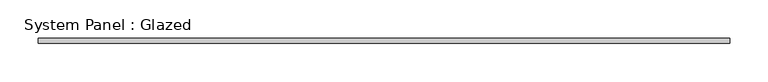
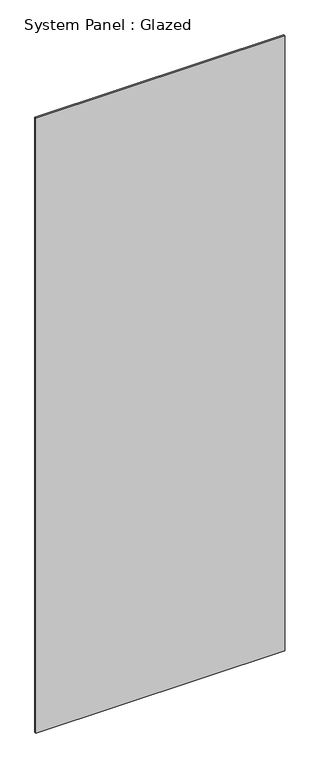
"""IFC4 building model written with IfcOpenShell, lengths in millimetres: plate geometry, System Panel : Glazed."""

from ifc_helpers import new_model, si_unit, origin, origin_with_axes, place, context, project, spatial, polyline, outline, extrude, source, transform, mapped, element, save


def system_panel_glazed_35c1503a(model_context):
    return source(origin(), model_context, "Body", "SweptSolid", [
        extrude(outline(polyline([(450.0, 34.0), (-450.0, 34.0), (-450.0, 40.0), (450.0, 40.0), (450.0, 34.0)])), origin_with_axes(), (0.0, 0.0, 1.0), 2350.0),
    ])


if __name__ == "__main__":
    model = new_model("IFC4")
    model_context = context("Model", 3, world=origin())
    ifc_project = project(units=[si_unit("LENGTHUNIT", "METRE", prefix="MILLI")], contexts=[model_context])
    site = spatial("IfcSite", under=ifc_project)
    building = spatial("IfcBuilding", under=site)
    placement = place(None, origin())
    system_panel_glazed_shape = system_panel_glazed_35c1503a(model_context)
    element("IfcPlate", 1, ObjectType="System Panel : Glazed", at=placement, inside=building, context=model_context, shape_type="MappedRepresentation", body=[
        mapped(system_panel_glazed_shape, transform((0.0, 0.0, 0.0), x_axis=(1.0, 0.0, 0.0), y_axis=(0.0, 1.0, 0.0), z_axis=(0.0, 0.0, 1.0))),
    ])
    save(model, "model.ifc")

# Revit data of these elements
# Type "System Panel : Glazed"
#   Construction Type Id = "GSP4R"
#   Analytic Construction = "1/8 in Pilkington single glazing"
#   Visual Light Transmittance = 0.9
#   Solar Heat Gain Coefficient = 0.86
#   Heat Transfer Coefficient (U) = 6.7069 W/(m²·K)
#   Define Thermal Properties by = 1
# Element 1 (IfcPlate, "System Panel : Glazed")
#   Materials on its faces: "Default New Material(6)"
# Materials
#   "Default New Material(6)": class "Generic", colour RGB 191 25 25, transparency 0.9, Cost = 0
